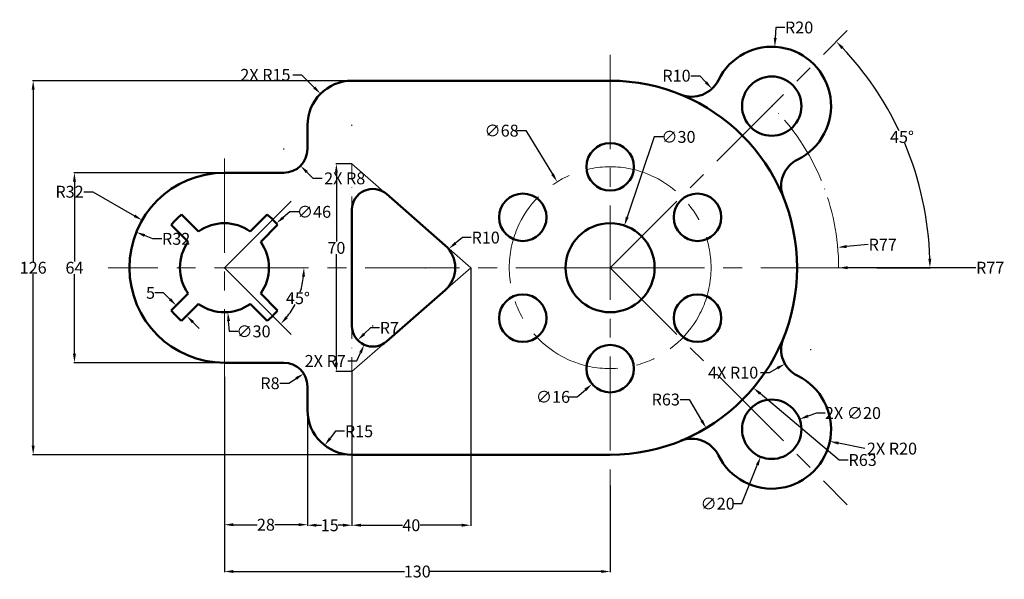
# Model space of a CAD drawing. Units: inches. Extents: x 234 to 566, y 84 to 273.
import ezdxf

# ---------------------------------------------------------------- set-up
doc = ezdxf.new("R2010")
doc.units = ezdxf.units.IN
doc.header["$MEASUREMENT"] = 0
doc.linetypes.add('ACAD_ISO04W100', pattern=[30, 24, -3, 0, -3])
doc.linetypes.add('CENTER', pattern=[50.8, 31.75, -6.35, 6.35, -6.35])
for name, color, linetype, lineweight in [('M-CNTR', 4, 'CENTER', 18), ('M-CONS', 4, 'ACAD_ISO04W100', 13), ('M-DIMS', 2, 'Continuous', 25), ('M-OUTL', 7, 'Continuous', 50)]:
    doc.layers.add(name, color=color, linetype=linetype, lineweight=lineweight)
doc.styles.get("Standard").update_dxf_attribs({"font": 'arial.ttf'})
doc.dimstyles.get("Standard").update_dxf_attribs({"dimtxt": 4, "dimasz": 3, "dimexe": 0.18, "dimexo": 0.0625, "dimgap": 0.09, "dimtad": 0, "dimtih": 1, "dimtoh": 1, "dimdec": 0, "dimzin": 0, "dimdsep": 46, "dimtxsty": 'Standard', "dimcen": 0.09, "dimadec": 0, "dimazin": 0, "dimtfac": 1, "dimtdec": 0, "dimtofl": 0, "dimtmove": 0, "dimatfit": 3, "dimfxl": 1, "dimtolj": 1, "dimtzin": 0, "dimarcsym": 0})

# ---------------------------------------------------------------- blocks, each defined once
blk = doc.blocks.new('*U1')
for p, q in [((-4.62, -1.09), (1.09, 4.62)), ((-1.09, -4.62), (4.62, 1.09))]:
    blk.add_line(p, q)
blk.add_arc((-13.31, -13.31), 23, 38.7599, 51.2401)
blk = doc.blocks.new('*U2')
at = {"layer": 'M-OUTL', "color": 0, "linetype": 'ByBlock', "lineweight": -2, "transparency": 16777216}
for p, rotation in [((289.46, 202.62), 90.00000000000003), ((289.46, 176), 180), ((316.09, 176), 270)]:
    blk.add_blockref('*U1', p, dxfattribs=dict(at, rotation=rotation))
blk.add_blockref('*U1', (316.09, 202.62), dxfattribs=at)
blk = doc.blocks.new('*D3')
at = {"layer": 'Defpoints', "color": 0, "transparency": 16777216}
for p in [(302.77, 152.6), (330.77, 149.31), (330.77, 102.72)]:
    blk.add_point(p, dxfattribs=at)
at = {"layer": 'M-DIMS', "color": 0, "lineweight": -2, "transparency": 16777216}
for p, q in [((302.77, 152.54), (302.77, 102.54)), ((330.77, 149.25), (330.77, 102.54)), ((305.77, 102.72), (313.78, 102.72)), ((327.77, 102.72), (319.77, 102.72))]:
    blk.add_line(p, q, dxfattribs=at)
at = {"layer": 'M-DIMS', "color": 0, "transparency": 16777216}
for points in [[(305.77, 103.22), (305.77, 102.22), (302.77, 102.72)], [(327.77, 103.22), (327.77, 102.22), (330.77, 102.72)]]:
    blk.add_solid(points, dxfattribs=at)
at = {"layer": 'M-DIMS', "color": 0, "transparency": 16777216, "insert": (316.77, 102.72), "char_height": 4, "attachment_point": 5}
blk.add_mtext('\\A1;28', dxfattribs=at)
blk = doc.blocks.new('*D4')
at = {"layer": 'Defpoints', "color": 0, "transparency": 16777216}
for p in [(302.77, 152.6), (432.77, 115.98), (432.77, 86.95)]:
    blk.add_point(p, dxfattribs=at)
at = {"layer": 'M-DIMS', "color": 0, "lineweight": -2, "transparency": 16777216}
for p, q in [((302.77, 152.54), (302.77, 86.77)), ((432.77, 115.92), (432.77, 86.77)), ((305.77, 86.95), (363.46, 86.95)), ((429.77, 86.95), (372.09, 86.95))]:
    blk.add_line(p, q, dxfattribs=at)
at = {"layer": 'M-DIMS', "color": 0, "transparency": 16777216}
for points in [[(305.77, 87.45), (305.77, 86.45), (302.77, 86.95)], [(429.77, 87.45), (429.77, 86.45), (432.77, 86.95)]]:
    blk.add_solid(points, dxfattribs=at)
at = {"layer": 'M-DIMS', "color": 0, "transparency": 16777216, "insert": (367.77, 86.95), "char_height": 4, "attachment_point": 5}
blk.add_mtext('\\A1;130', dxfattribs=at)
blk = doc.blocks.new('*D5')
at = {"layer": 'Defpoints', "color": 0, "transparency": 16777216}
for p in [(345.77, 252.31), (238.33, 126.31), (345.77, 126.31)]:
    blk.add_point(p, dxfattribs=at)
at = {"layer": 'M-DIMS', "color": 0, "lineweight": -2, "transparency": 16777216}
for p, q in [((345.71, 252.31), (238.15, 252.31)), ((238.33, 249.31), (238.33, 191.44)), ((238.33, 129.31), (238.33, 187.18)), ((345.71, 126.31), (238.15, 126.31))]:
    blk.add_line(p, q, dxfattribs=at)
at = {"layer": 'M-DIMS', "color": 0, "transparency": 16777216}
for points in [[(237.83, 249.31), (238.83, 249.31), (238.33, 252.31)], [(237.83, 129.31), (238.83, 129.31), (238.33, 126.31)]]:
    blk.add_solid(points, dxfattribs=at)
at = {"layer": 'M-DIMS', "color": 0, "transparency": 16777216, "insert": (238.33, 189.31), "char_height": 4, "attachment_point": 5}
blk.add_mtext('\\A1;126', dxfattribs=at)
blk = doc.blocks.new('*D6')
at = {"layer": 'Defpoints', "color": 0, "transparency": 16777216}
for p in [(302.77, 221.31), (252.24, 157.31), (302.77, 157.31)]:
    blk.add_point(p, dxfattribs=at)
at = {"layer": 'M-DIMS', "color": 0, "lineweight": -2, "transparency": 16777216}
for p, q in [((302.71, 221.31), (252.06, 221.31)), ((252.24, 218.31), (252.24, 191.44)), ((252.24, 160.31), (252.24, 187.18)), ((302.71, 157.31), (252.06, 157.31))]:
    blk.add_line(p, q, dxfattribs=at)
at = {"layer": 'M-DIMS', "color": 0, "transparency": 16777216}
for points in [[(251.74, 218.31), (252.74, 218.31), (252.24, 221.31)], [(251.74, 160.31), (252.74, 160.31), (252.24, 157.31)]]:
    blk.add_solid(points, dxfattribs=at)
at = {"layer": 'M-DIMS', "color": 0, "transparency": 16777216, "insert": (252.24, 189.31), "char_height": 4, "attachment_point": 5}
blk.add_mtext('\\A1;64', dxfattribs=at)
blk = doc.blocks.new('*D7')
at = {"layer": 'Defpoints', "color": 0, "transparency": 16777216}
for p in [(273.1, 201.29), (302.77, 189.31)]:
    blk.add_point(p, dxfattribs=at)
at = {"layer": 'M-DIMS', "color": 0, "lineweight": -2, "transparency": 16777216}
for p, q in [((278.66, 199.04), (275.88, 200.17)), ((281.66, 199.04), (278.66, 199.04))]:
    blk.add_line(p, q, dxfattribs=at)
at = {"layer": 'M-DIMS', "color": 0, "transparency": 16777216}
blk.add_solid([(276.07, 200.63), (275.7, 199.7), (273.1, 201.29)], dxfattribs=at)
at = {"layer": 'M-DIMS', "color": 0, "transparency": 16777216, "insert": (286.51, 199.04), "char_height": 4, "attachment_point": 5}
blk.add_mtext('\\A1;R32', dxfattribs=at)
blk = doc.blocks.new('*D8')
at = {"layer": 'Defpoints', "color": 0, "transparency": 16777216}
for p in [(320.27, 204.24), (285.28, 174.38)]:
    blk.add_point(p, dxfattribs=at)
at = {"layer": 'M-DIMS', "color": 0, "lineweight": -2, "transparency": 16777216}
for p, q in [((324.83, 208.13), (322.55, 206.19)), ((327.83, 208.13), (324.83, 208.13)), ((302.68, 189.31), (302.86, 189.31)), ((302.77, 189.22), (302.77, 189.4))]:
    blk.add_line(p, q, dxfattribs=at)
at = {"layer": 'M-DIMS', "color": 0, "transparency": 16777216}
blk.add_solid([(322.23, 206.57), (322.88, 205.81), (320.27, 204.24)], dxfattribs=at)
at = {"layer": 'M-DIMS', "color": 0, "transparency": 16777216, "insert": (332.96, 208.13), "char_height": 4, "attachment_point": 5}
blk.add_mtext('\\A1;∅46', dxfattribs=at)
blk = doc.blocks.new('*D9')
at = {"layer": 'Defpoints', "color": 0, "transparency": 16777216}
for p in [(301.61, 204.27), (303.94, 174.36)]:
    blk.add_point(p, dxfattribs=at)
at = {"layer": 'M-DIMS', "color": 0, "lineweight": -2, "transparency": 16777216}
for p, q in [((302.68, 189.31), (302.86, 189.31)), ((302.77, 189.22), (302.77, 189.4)), ((304.44, 167.85), (304.17, 171.36)), ((307.44, 167.85), (304.44, 167.85))]:
    blk.add_line(p, q, dxfattribs=at)
at = {"layer": 'M-DIMS', "color": 0, "transparency": 16777216}
blk.add_solid([(304.67, 171.4), (303.67, 171.33), (303.94, 174.36)], dxfattribs=at)
at = {"layer": 'M-DIMS', "color": 0, "transparency": 16777216, "insert": (312.57, 167.85), "char_height": 4, "attachment_point": 5}
blk.add_mtext('\\A1;∅30', dxfattribs=at)
blk = doc.blocks.new('*D10')
at = {"layer": 'Defpoints', "color": 0, "transparency": 16777216}
for p in [(286.53, 176.6), (284.84, 174.91), (288.37, 171.38)]:
    blk.add_point(p, dxfattribs=at)
at = {"layer": 'M-DIMS', "color": 0, "lineweight": -2, "transparency": 16777216}
for p, q in [((282.28, 180.84), (279.28, 180.84)), ((284.41, 178.72), (282.28, 180.84)), ((284.88, 174.96), (286.65, 176.73)), ((288.42, 171.42), (290.19, 173.19)), ((292.18, 170.94), (294.3, 168.82))]:
    blk.add_line(p, q, dxfattribs=at)
at = {"layer": 'M-DIMS', "color": 0, "transparency": 16777216}
for points in [[(284.76, 179.07), (284.05, 178.37), (286.53, 176.6)], [(292.54, 171.3), (291.83, 170.59), (290.06, 173.06)]]:
    blk.add_solid(points, dxfattribs=at)
at = {"layer": 'M-DIMS', "color": 0, "transparency": 16777216, "insert": (277.87, 180.84), "char_height": 4, "attachment_point": 5}
blk.add_mtext('\\A1;5', dxfattribs=at)
blk = doc.blocks.new('*D11')
at = {"layer": 'Defpoints', "color": 0, "transparency": 16777216}
for p in [(263.6, 189.31), (302.77, 189.31), (432.77, 189.31), (326.01, 175.9), (328.41, 163.67)]:
    blk.add_point(p, dxfattribs=at)
at = {"layer": 'M-DIMS', "color": 0, "lineweight": -2, "transparency": 16777216}
for start, end in [(342.3319, 353.5892), (321.4108, 332.4925)]:
    blk.add_arc((302.77, 189.31), 26.83, start, end, dxfattribs=at)
at = {"layer": 'M-DIMS', "color": 0, "transparency": 16777216}
for points in [[(328.93, 186.34), (329.93, 186.29), (329.6, 189.31)], [(324.12, 172.25), (323.37, 172.91), (321.74, 170.34)]]:
    blk.add_solid(points, dxfattribs=at)
at = {"layer": 'M-DIMS', "color": 0, "transparency": 16777216, "insert": (327.56, 179.04), "char_height": 4, "attachment_point": 5}
blk.add_mtext('\\A1;45°', dxfattribs=at)
blk = doc.blocks.new('*D12')
at = {"layer": 'Defpoints', "color": 0, "transparency": 16777216}
for p in [(330.77, 141.31), (345.77, 126.31), (345.77, 102.54)]:
    blk.add_point(p, dxfattribs=at)
at = {"layer": 'M-DIMS', "color": 0, "lineweight": -2, "transparency": 16777216}
for p, q in [((330.77, 141.25), (330.77, 102.36)), ((345.77, 126.25), (345.77, 102.36)), ((333.77, 102.54), (335.49, 102.54)), ((342.77, 102.54), (341.06, 102.54))]:
    blk.add_line(p, q, dxfattribs=at)
at = {"layer": 'M-DIMS', "color": 0, "transparency": 16777216}
for points in [[(333.77, 103.04), (333.77, 102.04), (330.77, 102.54)], [(342.77, 103.04), (342.77, 102.04), (345.77, 102.54)]]:
    blk.add_solid(points, dxfattribs=at)
at = {"layer": 'M-DIMS', "color": 0, "transparency": 16777216, "insert": (338.27, 102.54), "char_height": 4, "attachment_point": 5}
blk.add_mtext('\\A1;15', dxfattribs=at)
blk = doc.blocks.new('*D13')
at = {"layer": 'Defpoints', "color": 0, "transparency": 16777216}
for p in [(385.77, 189.31), (345.77, 154.31), (385.77, 102.54)]:
    blk.add_point(p, dxfattribs=at)
at = {"layer": 'M-DIMS', "color": 0, "lineweight": -2, "transparency": 16777216}
for p, q in [((385.77, 189.25), (385.77, 102.36)), ((345.77, 154.25), (345.77, 102.36)), ((348.77, 102.54), (362.75, 102.54)), ((382.77, 102.54), (368.8, 102.54))]:
    blk.add_line(p, q, dxfattribs=at)
at = {"layer": 'M-DIMS', "color": 0, "transparency": 16777216}
for points in [[(348.77, 103.04), (348.77, 102.04), (345.77, 102.54)], [(382.77, 103.04), (382.77, 102.04), (385.77, 102.54)]]:
    blk.add_solid(points, dxfattribs=at)
at = {"layer": 'M-DIMS', "color": 0, "transparency": 16777216, "insert": (365.77, 102.54), "char_height": 4, "attachment_point": 5}
blk.add_mtext('\\A1;40', dxfattribs=at)
blk = doc.blocks.new('*D14')
at = {"layer": 'Defpoints', "color": 0, "transparency": 16777216}
for p in [(345.77, 224.31), (340.51, 154.31), (345.77, 154.31)]:
    blk.add_point(p, dxfattribs=at)
at = {"layer": 'M-DIMS', "color": 0, "lineweight": -2, "transparency": 16777216}
for p, q in [((345.71, 224.31), (340.33, 224.31)), ((340.51, 221.31), (340.51, 198.12)), ((340.51, 157.31), (340.51, 193.85)), ((345.71, 154.31), (340.33, 154.31))]:
    blk.add_line(p, q, dxfattribs=at)
at = {"layer": 'M-DIMS', "color": 0, "transparency": 16777216}
for points in [[(340.01, 221.31), (341.01, 221.31), (340.51, 224.31)], [(340.01, 157.31), (341.01, 157.31), (340.51, 154.31)]]:
    blk.add_solid(points, dxfattribs=at)
at = {"layer": 'M-DIMS', "color": 0, "transparency": 16777216, "insert": (340.51, 195.99), "char_height": 4, "attachment_point": 5}
blk.add_mtext('\\A1;70', dxfattribs=at)
blk = doc.blocks.new('*D15')
at = {"layer": 'Defpoints', "color": 0, "transparency": 16777216}
for p in [(352.77, 169.74), (347.7, 164.91)]:
    blk.add_point(p, dxfattribs=at)
at = {"layer": 'M-DIMS', "color": 0, "lineweight": -2, "transparency": 16777216}
for p, q in [((352.05, 169.05), (349.88, 166.98)), ((355.05, 169.05), (352.05, 169.05))]:
    blk.add_line(p, q, dxfattribs=at)
at = {"layer": 'M-DIMS', "color": 0, "transparency": 16777216}
blk.add_solid([(349.53, 167.34), (350.22, 166.62), (347.7, 164.91)], dxfattribs=at)
at = {"layer": 'M-DIMS', "color": 0, "transparency": 16777216, "insert": (358.36, 169.05), "char_height": 4, "attachment_point": 5}
blk.add_mtext('\\A1;R7', dxfattribs=at)
blk = doc.blocks.new('*D16')
at = {"layer": 'Defpoints', "color": 0, "transparency": 16777216}
for p in [(378.32, 195.65), (370.59, 189.31)]:
    blk.add_point(p, dxfattribs=at)
at = {"layer": 'M-DIMS', "color": 0, "lineweight": -2, "transparency": 16777216}
for p, q in [((382.96, 199.46), (380.64, 197.56)), ((385.96, 199.46), (382.96, 199.46)), ((370.5, 189.31), (370.68, 189.31)), ((370.59, 189.22), (370.59, 189.4))]:
    blk.add_line(p, q, dxfattribs=at)
at = {"layer": 'M-DIMS', "color": 0, "transparency": 16777216}
blk.add_solid([(380.32, 197.94), (380.96, 197.17), (378.32, 195.65)], dxfattribs=at)
at = {"layer": 'M-DIMS', "color": 0, "transparency": 16777216, "insert": (390.82, 199.46), "char_height": 4, "attachment_point": 5}
blk.add_mtext('\\A1;R10', dxfattribs=at)
blk = doc.blocks.new('*U17')
blk.add_circle((0, 0), 8)
blk = doc.blocks.new('*U18')
at = {"layer": 'M-OUTL', "color": 0, "linetype": 'ByBlock', "lineweight": -2, "transparency": 16777216}
blk.add_blockref('*U17', (432.77, 223.31), dxfattribs=at)
for p, rotation in [((403.33, 206.31), 59.99999999999999), ((462.22, 206.31), 300), ((403.33, 172.31), 120), ((462.22, 172.31), 240), ((432.77, 155.31), 180)]:
    blk.add_blockref('*U17', p, dxfattribs=dict(at, rotation=rotation))
blk = doc.blocks.new('*D19')
at = {"layer": 'Defpoints', "color": 0, "transparency": 16777216}
for p in [(414.94, 218.26), (450.61, 160.36)]:
    blk.add_point(p, dxfattribs=at)
at = {"layer": 'M-DIMS', "color": 0, "lineweight": -2, "transparency": 16777216}
for p, q in [((401.32, 235.49), (404.32, 235.49)), ((404.32, 235.49), (413.36, 220.81)), ((432.68, 189.31), (432.86, 189.31)), ((432.77, 189.22), (432.77, 189.4))]:
    blk.add_line(p, q, dxfattribs=at)
at = {"layer": 'M-DIMS', "color": 0, "transparency": 16777216}
blk.add_solid([(413.79, 221.07), (412.94, 220.55), (414.94, 218.26)], dxfattribs=at)
at = {"layer": 'M-DIMS', "color": 0, "transparency": 16777216, "insert": (396.18, 235.49), "char_height": 4, "attachment_point": 5}
blk.add_mtext('\\A1;∅68', dxfattribs=at)
blk = doc.blocks.new('*D20')
at = {"layer": 'Defpoints', "color": 0, "transparency": 16777216}
for p in [(437.57, 203.52), (427.97, 175.1)]:
    blk.add_point(p, dxfattribs=at)
at = {"layer": 'M-DIMS', "color": 0, "lineweight": -2, "transparency": 16777216}
for p, q in [((447.66, 233.38), (438.53, 206.36)), ((450.66, 233.38), (447.66, 233.38)), ((432.68, 189.31), (432.86, 189.31)), ((432.77, 189.22), (432.77, 189.4))]:
    blk.add_line(p, q, dxfattribs=at)
at = {"layer": 'M-DIMS', "color": 0, "transparency": 16777216}
blk.add_solid([(438.06, 206.52), (439.01, 206.2), (437.57, 203.52)], dxfattribs=at)
at = {"layer": 'M-DIMS', "color": 0, "transparency": 16777216, "insert": (455.78, 233.38), "char_height": 4, "attachment_point": 5}
blk.add_mtext('\\A1;∅30', dxfattribs=at)
blk = doc.blocks.new('*D21')
at = {"layer": 'Defpoints', "color": 0, "transparency": 16777216}
for p in [(509.47, 196.18), (432.77, 189.31)]:
    blk.add_point(p, dxfattribs=at)
at = {"layer": 'M-DIMS', "color": 0, "lineweight": -2, "transparency": 16777216}
for p, q in [((519.75, 197.1), (512.46, 196.45)), ((432.68, 189.31), (432.86, 189.31)), ((432.77, 189.22), (432.77, 189.4))]:
    blk.add_line(p, q, dxfattribs=at)
at = {"layer": 'M-DIMS', "color": 0, "transparency": 16777216}
blk.add_solid([(512.41, 196.95), (512.5, 195.95), (509.47, 196.18)], dxfattribs=at)
at = {"layer": 'M-DIMS', "color": 0, "transparency": 16777216, "insert": (524.62, 197.1), "char_height": 4, "attachment_point": 5}
blk.add_mtext('\\A1;R77', dxfattribs=at)
blk = doc.blocks.new('*D22')
at = {"layer": 'Defpoints', "color": 0, "transparency": 16777216}
for p in [(512.68, 269.21), (536.86, 217.2), (432.77, 189.31), (432.77, 189.31), (522.62, 189.31)]:
    blk.add_point(p, dxfattribs=at)
at = {"layer": 'M-DIMS', "color": 0, "lineweight": -2, "transparency": 16777216}
blk.add_line((522.68, 189.31), (540.71, 189.31), dxfattribs=at)
for start, end in [(25.3655, 43.4048), (1.5952, 22.8903)]:
    blk.add_arc((432.77, 189.31), 107.76, start, end, dxfattribs=at)
at = {"layer": 'M-DIMS', "color": 0, "transparency": 16777216}
for points in [[(510.7, 263.01), (511.42, 263.7), (508.97, 265.51)], [(540.99, 192.32), (539.99, 192.3), (540.53, 189.31)]]:
    blk.add_solid(points, dxfattribs=at)
at = {"layer": 'M-DIMS', "color": 0, "transparency": 16777216, "insert": (531.12, 233.35), "char_height": 4, "attachment_point": 5}
blk.add_mtext('\\A1;45°', dxfattribs=at)
blk = doc.blocks.new('*D23')
at = {"layer": 'Defpoints', "color": 0, "transparency": 16777216}
for p in [(460.27, 256.93), (467.08, 249.61)]:
    blk.add_point(p, dxfattribs=at)
at = {"layer": 'M-DIMS', "color": 0, "lineweight": -2, "transparency": 16777216}
for p, q in [((459.99, 254.01), (462.99, 254.01)), ((462.99, 254.01), (465.04, 251.81))]:
    blk.add_line(p, q, dxfattribs=at)
at = {"layer": 'M-DIMS', "color": 0, "transparency": 16777216}
blk.add_solid([(465.4, 252.15), (464.67, 251.47), (467.08, 249.61)], dxfattribs=at)
at = {"layer": 'M-DIMS', "color": 0, "transparency": 16777216, "insert": (455.13, 254.01), "char_height": 4, "attachment_point": 5}
blk.add_mtext('\\A1;R10', dxfattribs=at)
blk = doc.blocks.new('*D24')
at = {"layer": 'Defpoints', "color": 0, "transparency": 16777216}
for p in [(488.25, 263.73), (487.22, 243.76)]:
    blk.add_point(p, dxfattribs=at)
at = {"layer": 'M-DIMS', "color": 0, "lineweight": -2, "transparency": 16777216}
for p, q in [((488.59, 270.25), (488.41, 266.73)), ((491.59, 270.25), (488.59, 270.25)), ((487.13, 243.76), (487.31, 243.76)), ((487.22, 243.67), (487.22, 243.85))]:
    blk.add_line(p, q, dxfattribs=at)
at = {"layer": 'M-DIMS', "color": 0, "transparency": 16777216}
blk.add_solid([(487.91, 266.75), (488.9, 266.7), (488.25, 263.73)], dxfattribs=at)
at = {"layer": 'M-DIMS', "color": 0, "transparency": 16777216, "insert": (496.45, 270.25), "char_height": 4, "attachment_point": 5}
blk.add_mtext('\\A1;R20', dxfattribs=at)
blk = doc.blocks.new('*D25')
at = {"layer": 'Defpoints', "color": 0, "transparency": 16777216}
for p in [(432.77, 189.31), (465.15, 135.26)]:
    blk.add_point(p, dxfattribs=at)
at = {"layer": 'M-DIMS', "color": 0, "lineweight": -2, "transparency": 16777216}
for p, q in [((456.38, 144.9), (459.38, 144.9)), ((459.38, 144.9), (463.61, 137.84))]:
    blk.add_line(p, q, dxfattribs=at)
at = {"layer": 'M-DIMS', "color": 0, "transparency": 16777216}
blk.add_solid([(464.03, 138.1), (463.18, 137.58), (465.15, 135.26)], dxfattribs=at)
at = {"layer": 'M-DIMS', "color": 0, "transparency": 16777216, "insert": (451.51, 144.9), "char_height": 4, "attachment_point": 5}
blk.add_mtext('\\A1;R63', dxfattribs=at)
blk = doc.blocks.new('*D26')
at = {"layer": 'Defpoints', "color": 0, "transparency": 16777216}
for p in [(438.86, 160.51), (426.69, 150.12)]:
    blk.add_point(p, dxfattribs=at)
at = {"layer": 'M-DIMS', "color": 0, "lineweight": -2, "transparency": 16777216}
for p, q in [((432.68, 155.31), (432.86, 155.31)), ((432.77, 155.22), (432.77, 155.4)), ((421.63, 145.79), (424.41, 148.17)), ((418.63, 145.79), (421.63, 145.79))]:
    blk.add_line(p, q, dxfattribs=at)
at = {"layer": 'M-DIMS', "color": 0, "transparency": 16777216}
blk.add_solid([(424.08, 148.55), (424.73, 147.79), (426.69, 150.12)], dxfattribs=at)
at = {"layer": 'M-DIMS', "color": 0, "transparency": 16777216, "insert": (413.5, 145.79), "char_height": 4, "attachment_point": 5}
blk.add_mtext('\\A1;∅16', dxfattribs=at)
blk = doc.blocks.new('*D27')
at = {"layer": 'Defpoints', "color": 0, "transparency": 16777216}
for p in [(329.51, 153.63), (322.77, 149.31)]:
    blk.add_point(p, dxfattribs=at)
at = {"layer": 'M-DIMS', "color": 0, "lineweight": -2, "transparency": 16777216}
for p, q in [((321.46, 150.39), (324.46, 150.39)), ((324.46, 150.39), (326.98, 152.01))]:
    blk.add_line(p, q, dxfattribs=at)
at = {"layer": 'M-DIMS', "color": 0, "transparency": 16777216}
blk.add_solid([(326.71, 152.43), (327.25, 151.59), (329.51, 153.63)], dxfattribs=at)
at = {"layer": 'M-DIMS', "color": 0, "transparency": 16777216, "insert": (318.14, 150.39), "char_height": 4, "attachment_point": 5}
blk.add_mtext('\\A1;R8', dxfattribs=at)
blk = doc.blocks.new('*D28')
at = {"layer": 'Defpoints', "color": 0, "transparency": 16777216}
for p in [(345.77, 141.31), (336.57, 129.47)]:
    blk.add_point(p, dxfattribs=at)
at = {"layer": 'M-DIMS', "color": 0, "lineweight": -2, "transparency": 16777216}
for p, q in [((340.25, 134.2), (338.41, 131.84)), ((343.25, 134.2), (340.25, 134.2))]:
    blk.add_line(p, q, dxfattribs=at)
at = {"layer": 'M-DIMS', "color": 0, "transparency": 16777216}
blk.add_solid([(338.02, 132.14), (338.81, 131.53), (336.57, 129.47)], dxfattribs=at)
at = {"layer": 'M-DIMS', "color": 0, "transparency": 16777216, "insert": (348.14, 134.2), "char_height": 4, "attachment_point": 5}
blk.add_mtext('\\A1;R15', dxfattribs=at)
blk = doc.blocks.new('*D29')
at = {"layer": 'Defpoints', "color": 0, "transparency": 16777216}
for p in [(490.96, 144.14), (483.48, 125.59)]:
    blk.add_point(p, dxfattribs=at)
at = {"layer": 'M-DIMS', "color": 0, "lineweight": -2, "transparency": 16777216}
for p, q in [((487.13, 134.86), (487.31, 134.86)), ((487.22, 134.77), (487.22, 134.95)), ((477.11, 109.81), (482.36, 122.81)), ((474.11, 109.81), (477.11, 109.81))]:
    blk.add_line(p, q, dxfattribs=at)
at = {"layer": 'M-DIMS', "color": 0, "transparency": 16777216}
blk.add_solid([(481.89, 122.99), (482.82, 122.62), (483.48, 125.59)], dxfattribs=at)
at = {"layer": 'M-DIMS', "color": 0, "transparency": 16777216, "insert": (468.99, 109.81), "char_height": 4, "attachment_point": 5}
blk.add_mtext('\\A1;∅20', dxfattribs=at)
blk = doc.blocks.new('PLATE-LUG-D20')
blk.add_circle((0, 0), 10)
for centre, radius, start, end in [((0, 0), 20, 296.0541, 153.9459), ((-26.95, 13.18), 10, 247.8733, 333.9459), ((13.18, -26.95), 10, 116.0541, 202.1267)]:
    blk.add_arc(centre, radius, start, end)
blk = doc.blocks.new('*D31')
at = {"layer": 'Defpoints', "color": 0, "transparency": 16777216}
for p in [(275.06, 205.31), (302.77, 189.31)]:
    blk.add_point(p, dxfattribs=at)
at = {"layer": 'M-DIMS', "color": 0, "lineweight": -2, "transparency": 16777216}
for p, q in [((255.43, 214.91), (258.43, 214.91)), ((258.43, 214.91), (272.46, 206.81)), ((302.68, 189.31), (302.86, 189.31)), ((302.77, 189.22), (302.77, 189.4))]:
    blk.add_line(p, q, dxfattribs=at)
at = {"layer": 'M-DIMS', "color": 0, "transparency": 16777216}
blk.add_solid([(272.71, 207.24), (272.21, 206.38), (275.06, 205.31)], dxfattribs=at)
at = {"layer": 'M-DIMS', "color": 0, "transparency": 16777216, "insert": (250.58, 214.91), "char_height": 4, "attachment_point": 5}
blk.add_mtext('\\A1;R32', dxfattribs=at)
blk = doc.blocks.new('*D32')
at = {"layer": 'Defpoints', "color": 0, "transparency": 16777216}
for p in [(322.77, 229.31), (328.43, 223.65)]:
    blk.add_point(p, dxfattribs=at)
at = {"layer": 'M-DIMS', "color": 0, "lineweight": -2, "transparency": 16777216}
for p, q in [((322.68, 229.31), (322.86, 229.31)), ((322.77, 229.22), (322.77, 229.4)), ((332.67, 219.41), (330.55, 221.53)), ((335.67, 219.41), (332.67, 219.41))]:
    blk.add_line(p, q, dxfattribs=at)
at = {"layer": 'M-DIMS', "color": 0, "transparency": 16777216}
blk.add_solid([(330.91, 221.89), (330.2, 221.18), (328.43, 223.65)], dxfattribs=at)
at = {"layer": 'M-DIMS', "color": 0, "transparency": 16777216, "insert": (343.32, 219.41), "char_height": 4, "attachment_point": 5}
blk.add_mtext('\\A1;2X R8', dxfattribs=at)
blk = doc.blocks.new('*D33')
at = {"layer": 'Defpoints', "color": 0, "transparency": 16777216}
for p in [(335.17, 247.92), (345.77, 237.31)]:
    blk.add_point(p, dxfattribs=at)
at = {"layer": 'M-DIMS', "color": 0, "lineweight": -2, "transparency": 16777216}
for p, q in [((325.81, 254.29), (328.81, 254.29)), ((328.81, 254.29), (333.05, 250.04)), ((345.68, 237.31), (345.86, 237.31)), ((345.77, 237.22), (345.77, 237.4))]:
    blk.add_line(p, q, dxfattribs=at)
at = {"layer": 'M-DIMS', "color": 0, "transparency": 16777216}
blk.add_solid([(333.4, 250.4), (332.7, 249.69), (335.17, 247.92)], dxfattribs=at)
at = {"layer": 'M-DIMS', "color": 0, "transparency": 16777216, "insert": (316.59, 254.29), "char_height": 4, "attachment_point": 5}
blk.add_mtext('\\A1;2X R15', dxfattribs=at)
blk = doc.blocks.new('*D34')
at = {"layer": 'Defpoints', "color": 0, "transparency": 16777216}
for p in [(352.77, 169.74), (349.88, 163.36)]:
    blk.add_point(p, dxfattribs=at)
at = {"layer": 'M-DIMS', "color": 0, "lineweight": -2, "transparency": 16777216}
for p, q in [((352.68, 169.74), (352.86, 169.74)), ((352.77, 169.65), (352.77, 169.83)), ((347.4, 157.9), (348.64, 160.63)), ((344.4, 157.9), (347.4, 157.9))]:
    blk.add_line(p, q, dxfattribs=at)
at = {"layer": 'M-DIMS', "color": 0, "transparency": 16777216}
blk.add_solid([(348.19, 160.84), (349.1, 160.42), (349.88, 163.36)], dxfattribs=at)
at = {"layer": 'M-DIMS', "color": 0, "transparency": 16777216, "insert": (336.76, 157.9), "char_height": 4, "attachment_point": 5}
blk.add_mtext('\\A1;2X R7', dxfattribs=at)
blk = doc.blocks.new('*D35')
at = {"layer": 'Defpoints', "color": 0, "transparency": 16777216}
for p in [(432.77, 189.31), (481.03, 148.81)]:
    blk.add_point(p, dxfattribs=at)
at = {"layer": 'M-DIMS', "color": 0, "lineweight": -2, "transparency": 16777216}
for p, q in [((432.68, 189.31), (432.86, 189.31)), ((432.77, 189.22), (432.77, 189.4)), ((509.99, 124.52), (483.33, 146.89)), ((512.99, 124.52), (509.99, 124.52))]:
    blk.add_line(p, q, dxfattribs=at)
at = {"layer": 'M-DIMS', "color": 0, "transparency": 16777216}
blk.add_solid([(483.65, 147.27), (483.01, 146.5), (481.03, 148.81)], dxfattribs=at)
at = {"layer": 'M-DIMS', "color": 0, "transparency": 16777216, "insert": (517.86, 124.52), "char_height": 4, "attachment_point": 5}
blk.add_mtext('\\A1;R63', dxfattribs=at)
blk = doc.blocks.new('*D36')
at = {"layer": 'Defpoints', "color": 0, "transparency": 16777216}
for p in [(500.4, 161.81), (491.69, 156.91)]:
    blk.add_point(p, dxfattribs=at)
at = {"layer": 'M-DIMS', "color": 0, "lineweight": -2, "transparency": 16777216}
for p, q in [((500.31, 161.81), (500.49, 161.81)), ((500.4, 161.72), (500.4, 161.9)), ((483.46, 153.96), (486.46, 153.96)), ((486.46, 153.96), (489.07, 155.43))]:
    blk.add_line(p, q, dxfattribs=at)
at = {"layer": 'M-DIMS', "color": 0, "transparency": 16777216}
blk.add_solid([(488.83, 155.87), (489.32, 155), (491.69, 156.91)], dxfattribs=at)
at = {"layer": 'M-DIMS', "color": 0, "transparency": 16777216, "insert": (474.22, 153.96), "char_height": 4, "attachment_point": 5}
blk.add_mtext('\\A1;4X R10', dxfattribs=at)
blk = doc.blocks.new('*D37')
at = {"layer": 'Defpoints', "color": 0, "transparency": 16777216}
for p in [(432.77, 189.31), (509.77, 189.31)]:
    blk.add_point(p, dxfattribs=at)
at = {"layer": 'M-DIMS', "color": 0, "lineweight": -2, "transparency": 16777216}
for p, q in [((432.68, 189.31), (432.86, 189.31)), ((432.77, 189.22), (432.77, 189.4)), ((555.97, 189.31), (512.77, 189.31))]:
    blk.add_line(p, q, dxfattribs=at)
at = {"layer": 'M-DIMS', "color": 0, "transparency": 16777216}
blk.add_solid([(512.77, 189.81), (512.77, 188.81), (509.77, 189.31)], dxfattribs=at)
at = {"layer": 'M-DIMS', "color": 0, "transparency": 16777216, "insert": (560.84, 189.31), "char_height": 4, "attachment_point": 5}
blk.add_mtext('\\A1;R77', dxfattribs=at)
blk = doc.blocks.new('*D38')
at = {"layer": 'Defpoints', "color": 0, "transparency": 16777216}
for p in [(487.22, 134.86), (506.8, 130.8)]:
    blk.add_point(p, dxfattribs=at)
at = {"layer": 'M-DIMS', "color": 0, "lineweight": -2, "transparency": 16777216}
for p, q in [((487.13, 134.86), (487.31, 134.86)), ((487.22, 134.77), (487.22, 134.95)), ((518.55, 128.36), (509.74, 130.19))]:
    blk.add_line(p, q, dxfattribs=at)
at = {"layer": 'M-DIMS', "color": 0, "transparency": 16777216}
blk.add_solid([(509.84, 130.68), (509.64, 129.7), (506.8, 130.8)], dxfattribs=at)
at = {"layer": 'M-DIMS', "color": 0, "transparency": 16777216, "insert": (527.75, 128.36), "char_height": 4, "attachment_point": 5}
blk.add_mtext('\\A1;2X R20', dxfattribs=at)
blk = doc.blocks.new('*D39')
at = {"layer": 'Defpoints', "color": 0, "transparency": 16777216}
for p in [(496.62, 138.29), (477.83, 131.44)]:
    blk.add_point(p, dxfattribs=at)
at = {"layer": 'M-DIMS', "color": 0, "lineweight": -2, "transparency": 16777216}
for p, q in [((502.26, 140.34), (499.44, 139.31)), ((505.26, 140.34), (502.26, 140.34)), ((487.13, 134.86), (487.31, 134.86)), ((487.22, 134.77), (487.22, 134.95))]:
    blk.add_line(p, q, dxfattribs=at)
at = {"layer": 'M-DIMS', "color": 0, "transparency": 16777216}
blk.add_solid([(499.27, 139.78), (499.61, 138.84), (496.62, 138.29)], dxfattribs=at)
at = {"layer": 'M-DIMS', "color": 0, "transparency": 16777216, "insert": (514.6, 140.34), "char_height": 4, "attachment_point": 5}
blk.add_mtext('\\A1;2X ∅20', dxfattribs=at)

msp = doc.modelspace()

# ---------------------------------------------------------------- linework, layer by layer
at = {"layer": 'M-CNTR'}
for p, q in [((432.77, 189.31), (512.68, 269.21)), ((432.77, 261.03), (432.77, 115.98)), ((302.77, 226.1), (302.77, 152.6)), ((302.77, 189.31), (328.71, 215.25)), ((432.77, 189.31), (263.6, 189.31)), ((302.77, 189.31), (328.41, 163.67)), ((432.77, 189.31), (512.68, 109.41)), ((432.77, 189.31), (522.62, 189.31))]:
    msp.add_line(p, q, dxfattribs=at)
msp.add_circle((432.77, 189.31), 34, dxfattribs=at)
at = {"layer": 'M-CONS'}
for p, q in [((345.77, 189.31), (345.77, 224.31)), ((345.77, 224.31), (385.77, 189.31)), ((345.77, 189.31), (345.77, 154.31)), ((345.77, 154.31), (385.77, 189.31))]:
    msp.add_line(p, q, dxfattribs=at)
msp.add_arc((432.77, 189.31), 77, 0, 45, dxfattribs=at)
at = {"layer": 'M-OUTL'}
for p, q in [((432.77, 252.31), (345.77, 252.31)), ((330.77, 229.31), (330.77, 237.31)), ((302.77, 221.31), (322.77, 221.31)), ((357.38, 214.15), (377.17, 196.84)), ((345.77, 189.31), (345.77, 208.88)), ((345.77, 189.31), (345.77, 169.74)), ((357.38, 164.47), (377.17, 181.79)), ((302.77, 157.31), (322.77, 157.31)), ((330.77, 149.31), (330.77, 141.31)), ((432.77, 126.31), (345.77, 126.31))]:
    msp.add_line(p, q, dxfattribs=at)
msp.add_circle((432.77, 189.31), 15, dxfattribs=at)
for centre, radius, start, end in [((345.77, 237.31), 15, 90, 180), ((432.77, 189.31), 63, 270, 90), ((322.77, 229.31), 8, 270, 0), ((302.77, 189.31), 32, 90, 270), ((352.77, 208.88), 7, 48.8141, 180), ((302.77, 189.31), 15, 54.5941, 125.4059), ((302.77, 189.31), 15, 144.5941, 215.4059), ((302.77, 189.31), 15, 324.5941, 35.4059), ((370.59, 189.31), 10, 311.1859, 48.8141), ((302.77, 189.31), 15, 234.5941, 305.4059), ((352.77, 169.74), 7, 180, 311.1859), ((322.77, 149.31), 8, 0, 90), ((345.77, 141.31), 15, 180, 270)]:
    msp.add_arc(centre, radius, start, end, dxfattribs=at)

# ---------------------------------------------------------------- block references
for name, p in [('PLATE-LUG-D20', (487.22, 243.76)), ('*U18', (0, 0)), ('*U2', (0, 0))]:
    msp.add_blockref(name, p, dxfattribs=at)
at = {"layer": 'M-OUTL', "rotation": 270.0000000000001}
msp.add_blockref('PLATE-LUG-D20', (487.22, 134.86), dxfattribs=at)

# ---------------------------------------------------------------- dimensions: what is measured, and where the dimension line sits
at = {"layer": 'M-DIMS'}
for center, mpoint, override, picture, middle in [((487.22, 243.76), (488.25, 263.73), {"dimclrd": 0, "dimclre": 0, "dimclrt": 0}, '*D24', (496.45, 270.25)), ((460.27, 256.93), (467.08, 249.61), {"dimclrd": 0, "dimclre": 0, "dimclrt": 0}, '*D23', (455.13, 254.01)), ((302.77, 189.31), (275.06, 205.31), {"dimdec": 0, "dimlfac": 1, "dimrnd": 0, "dimzin": 0, "dimdsep": 46, "dimlunit": 2}, '*D31', (250.58, 214.91)), ((302.77, 189.31), (273.1, 201.29), {"dimclrd": 0, "dimclre": 0, "dimclrt": 0}, '*D7', (286.51, 199.04)), ((432.77, 189.31), (509.47, 196.18), {"dimclrd": 0, "dimclre": 0, "dimclrt": 0}, '*D21', (519.75, 197.1)), ((432.77, 189.31), (509.77, 189.31), {"dimdec": 0, "dimlfac": 1, "dimrnd": 0, "dimzin": 0, "dimdsep": 46, "dimlunit": 2}, '*D37', (555.97, 189.31)), ((432.77, 189.31), (481.03, 148.81), {"dimdec": 0, "dimlfac": 1, "dimrnd": 0, "dimzin": 0, "dimdsep": 46, "dimlunit": 2}, '*D35', (517.86, 124.52)), ((432.77, 189.31), (465.15, 135.26), {"dimclrd": 0, "dimclre": 0, "dimclrt": 0}, '*D25', (451.51, 144.9)), ((352.77, 169.74), (347.7, 164.91), {"dimclrd": 0, "dimclre": 0, "dimclrt": 0}, '*D15', (358.36, 169.05)), ((322.77, 149.31), (329.51, 153.63), {"dimclrd": 0, "dimclre": 0, "dimclrt": 0}, '*D27', (318.14, 150.39)), ((345.77, 141.31), (336.57, 129.47), {"dimclrd": 0, "dimclre": 0, "dimclrt": 0}, '*D28', (348.14, 134.2))]:
    dim = msp.add_radius_dim(center=center, mpoint=mpoint, dimstyle='Standard', override=override, dxfattribs=at)
    dim.commit()
    dim.dimension.update_dxf_attribs({"geometry": picture, "text_midpoint": middle, "dimtype": 164})
dim = msp.add_angular_dim_2l(base=(536.86, 217.2), line1=((432.77, 189.31), (522.62, 189.31)), line2=((432.77, 189.31), (512.68, 269.21)), dimstyle='Standard', override={"dimclrd": 0, "dimclre": 0, "dimclrt": 0}, dxfattribs=at)
dim.commit()
dim.dimension.update_dxf_attribs({"geometry": '*D22', "text_midpoint": (531.12, 233.35), "dimtype": 162})
for center, mpoint, text, picture, middle in [((345.77, 237.31), (335.17, 247.92), '2X <>', '*D33', (316.59, 254.29)), ((500.4, 161.81), (491.69, 156.91), '4X <>', '*D36', (474.22, 153.96)), ((487.22, 134.86), (506.8, 130.8), '2X <>', '*D38', (518.55, 128.36))]:
    dim = msp.add_radius_dim(center=center, mpoint=mpoint, text=text, dimstyle='Standard', override={"dimdec": 0, "dimlfac": 1, "dimrnd": 0, "dimzin": 0, "dimdsep": 46, "dimlunit": 2}, dxfattribs=at)
    dim.commit()
    dim.dimension.update_dxf_attribs({"geometry": picture, "text_midpoint": middle, "dimtype": 164})
for base, p1, p2, picture, middle in [((238.33, 126.31), (345.77, 252.31), (345.77, 126.31), '*D5', (238.33, 189.31)), ((252.24, 157.31), (302.77, 221.31), (302.77, 157.31), '*D6', (252.24, 189.31))]:
    dim = msp.add_linear_dim(base=base, p1=p1, p2=p2, angle=90, dimstyle='Standard', override={"dimclrd": 0, "dimclre": 0, "dimclrt": 0}, dxfattribs=at)
    dim.commit()
    dim.dimension.update_dxf_attribs({"geometry": picture, "text_midpoint": middle})
for p1, p2, picture, middle in [((450.61, 160.36), (414.94, 218.26), '*D19', (396.18, 235.49)), ((427.97, 175.1), (437.57, 203.52), '*D20', (455.78, 233.38)), ((301.61, 204.27), (303.94, 174.36), '*D9', (312.57, 167.85)), ((438.86, 160.51), (426.69, 150.12), '*D26', (413.5, 145.79)), ((490.96, 144.14), (483.48, 125.59), '*D29', (468.99, 109.81))]:
    dim = msp.add_diameter_dim_2p(p1=p1, p2=p2, dimstyle='Standard', override={"dimclrd": 0, "dimclre": 0, "dimclrt": 0}, dxfattribs=at)
    dim.commit()
    dim.dimension.update_dxf_attribs({"geometry": picture, "text_midpoint": middle, "dimtype": 163})
for center, mpoint, picture, middle in [((322.77, 229.31), (328.43, 223.65), '*D32', (343.32, 219.41)), ((352.77, 169.74), (349.88, 163.36), '*D34', (336.76, 157.9))]:
    dim = msp.add_radius_dim(center=center, mpoint=mpoint, text='2X <>', dimstyle='Standard', override={"dimdec": 0, "dimlfac": 1, "dimrnd": 0, "dimzin": 0, "dimdsep": 46, "dimlunit": 2}, dxfattribs=at)
    dim.commit()
    dim.dimension.update_dxf_attribs({"geometry": picture, "text_midpoint": middle})
dim = msp.add_linear_dim(base=(340.51, 154.31), p1=(345.77, 224.31), p2=(345.77, 154.31), angle=90, dimstyle='Standard', override={"dimclrd": 0, "dimclre": 0, "dimclrt": 0}, dxfattribs=at)
dim.commit()
dim.dimension.update_dxf_attribs({"geometry": '*D14', "text_midpoint": (340.51, 195.99), "dimtype": 160})
dim = msp.add_diameter_dim_2p(p1=(285.28, 174.38), p2=(320.27, 204.24), dimstyle='Standard', override={"dimclrd": 0, "dimclre": 0, "dimclrt": 0}, dxfattribs=at)
dim.commit()
dim.dimension.update_dxf_attribs({"geometry": '*D8', "text_midpoint": (332.96, 208.13)})
dim = msp.add_radius_dim(center=(370.59, 189.31), mpoint=(378.32, 195.65), dimstyle='Standard', override={"dimclrd": 0, "dimclre": 0, "dimclrt": 0}, dxfattribs=at)
dim.commit()
dim.dimension.update_dxf_attribs({"geometry": '*D16', "text_midpoint": (390.82, 199.46)})
dim = msp.add_angular_dim_2l(base=(326.01, 175.9), line1=((302.77, 189.31), (328.41, 163.67)), line2=((432.77, 189.31), (263.6, 189.31)), dimstyle='Standard', override={"dimclrd": 0, "dimclre": 0, "dimclrt": 0}, dxfattribs=at)
dim.commit()
dim.dimension.update_dxf_attribs({"geometry": '*D11', "text_midpoint": (327.56, 179.04)})
for base, p1, p2, picture, middle in [((385.77, 102.54), (345.77, 154.31), (385.77, 189.31), '*D13', (365.77, 102.54)), ((330.77, 102.72), (302.77, 152.6), (330.77, 149.31), '*D3', (316.77, 102.72)), ((432.77, 86.95), (302.77, 152.6), (432.77, 115.98), '*D4', (367.77, 86.95)), ((345.77, 102.54), (330.77, 141.31), (345.77, 126.31), '*D12', (338.27, 102.54))]:
    dim = msp.add_linear_dim(base=base, p1=p1, p2=p2, dimstyle='Standard', override={"dimclrd": 0, "dimclre": 0, "dimclrt": 0}, dxfattribs=at)
    dim.commit()
    dim.dimension.update_dxf_attribs({"geometry": picture, "text_midpoint": middle})
dim = msp.add_aligned_dim(p1=(288.37, 171.38), p2=(284.84, 174.91), distance=-2.39, dimstyle='Standard', override={"dimclrd": 0, "dimclre": 0, "dimclrt": 0}, dxfattribs=at)
dim.commit()
dim.dimension.update_dxf_attribs({"geometry": '*D10', "text_midpoint": (277.87, 180.84)})
dim = msp.add_diameter_dim_2p(p1=(477.83, 131.44), p2=(496.62, 138.29), text='2X <>', dimstyle='Standard', override={"dimdec": 0, "dimlfac": 1, "dimrnd": 0, "dimzin": 0, "dimdsep": 46, "dimlunit": 2}, dxfattribs=at)
dim.commit()
dim.dimension.update_dxf_attribs({"geometry": '*D39', "text_midpoint": (514.6, 140.34), "dimtype": 163})

doc.saveas('drawing.dxf')
